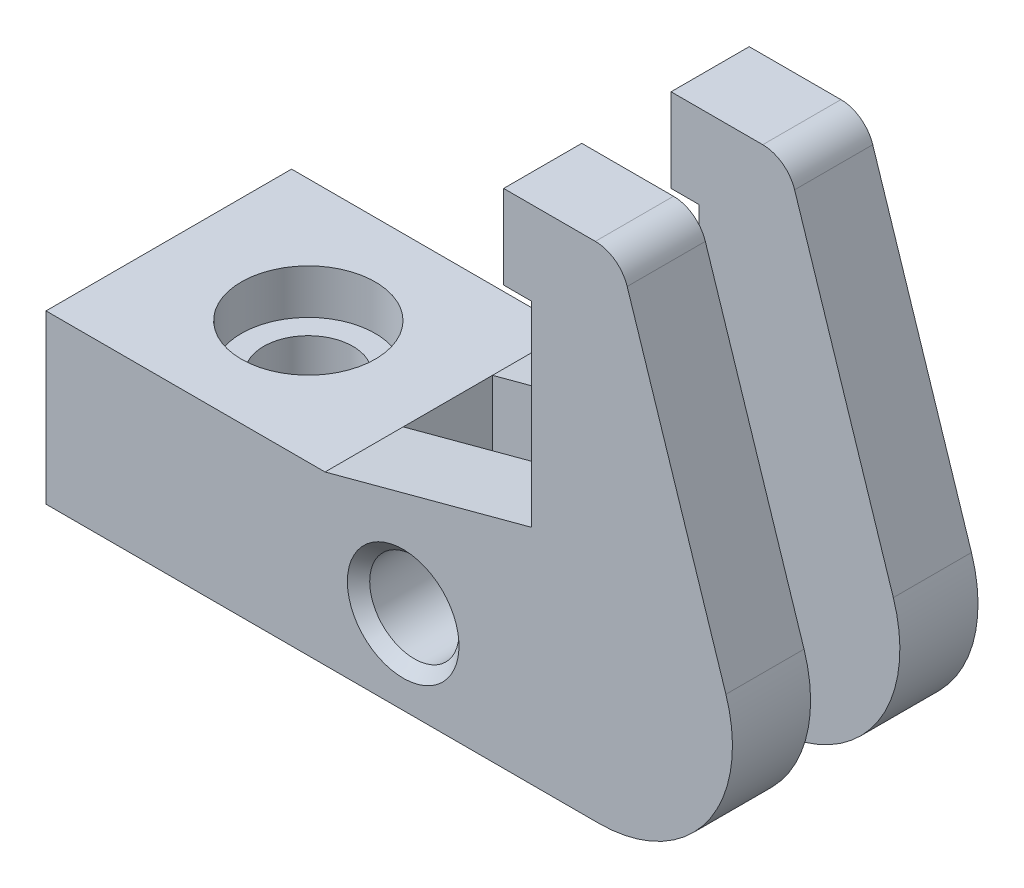
ISO-10303-21;
HEADER;
FILE_DESCRIPTION(('STEP AP214'),'2;1');
FILE_NAME('part.step','',(''),(''),'','','');
FILE_SCHEMA(('AUTOMOTIVE_DESIGN { 1 0 10303 214 1 1 1 1 }'));
ENDSEC;
DATA;
#1=APPLICATION_CONTEXT('core data for automotive mechanical design processes');
#2=APPLICATION_PROTOCOL_DEFINITION('international standard','automotive_design',2000,#1);
#3=PRODUCT_CONTEXT('',#1,'mechanical');
#4=PRODUCT('Part','Part','',(#3));
#5=PRODUCT_RELATED_PRODUCT_CATEGORY('part','',(#4));
#6=PRODUCT_DEFINITION_FORMATION('','',#4);
#7=PRODUCT_DEFINITION_CONTEXT('part definition',#1,'design');
#8=PRODUCT_DEFINITION('design','',#6,#7);
#9=PRODUCT_DEFINITION_SHAPE('','',#8);
#10=(LENGTH_UNIT() NAMED_UNIT(*) SI_UNIT(.MILLI.,.METRE.));
#11=(NAMED_UNIT(*) PLANE_ANGLE_UNIT() SI_UNIT($,.RADIAN.));
#12=(NAMED_UNIT(*) SI_UNIT($,.STERADIAN.) SOLID_ANGLE_UNIT());
#13=UNCERTAINTY_MEASURE_WITH_UNIT(LENGTH_MEASURE(1.E-05),#10,'distance_accuracy_value','');
#14=(GEOMETRIC_REPRESENTATION_CONTEXT(3) GLOBAL_UNCERTAINTY_ASSIGNED_CONTEXT((#13)) GLOBAL_UNIT_ASSIGNED_CONTEXT((#10,
#11,#12)) REPRESENTATION_CONTEXT('',''));
#15=CARTESIAN_POINT('',(0.,0.,0.));
#16=DIRECTION('',(0.,0.,1.));
#17=DIRECTION('',(1.,0.,0.));
#18=AXIS2_PLACEMENT_3D('',#15,#16,#17);
#19=CARTESIAN_POINT('',(32.,0.,11.));
#20=DIRECTION('',(0.,1.,0.));
#21=DIRECTION('',(0.,0.,1.));
#22=AXIS2_PLACEMENT_3D('',#19,#20,#21);
#23=PLANE('',#22);
#24=CARTESIAN_POINT('',(12.5,0.,0.));
#25=DIRECTION('',(0.,1.,0.));
#26=DIRECTION('',(0.,0.,1.));
#27=AXIS2_PLACEMENT_3D('',#24,#25,#26);
#28=CIRCLE('',#27,4.00000000000001);
#29=CARTESIAN_POINT('',(12.5,0.,4.00000000000001));
#30=VERTEX_POINT('',#29);
#31=EDGE_CURVE('E459',#30,#30,#28,.T.);
#32=ORIENTED_EDGE('',*,*,#31,.T.);
#33=EDGE_LOOP('',(#32));
#34=FACE_BOUND('',#33,.T.);
#35=DIRECTION('',(1.,0.,0.));
#36=VECTOR('',#35,1.);
#37=CARTESIAN_POINT('',(25.,0.,4.));
#38=LINE('',#37,#36);
#39=CARTESIAN_POINT('',(25.,0.,4.));
#40=VERTEX_POINT('',#39);
#41=CARTESIAN_POINT('',(49.5,0.,4.));
#42=VERTEX_POINT('',#41);
#43=EDGE_CURVE('E309',#40,#42,#38,.T.);
#44=ORIENTED_EDGE('',*,*,#43,.T.);
#45=DIRECTION('',(0.,0.,-1.));
#46=VECTOR('',#45,1.);
#47=CARTESIAN_POINT('',(49.5,0.,11.));
#48=LINE('',#47,#46);
#49=CARTESIAN_POINT('',(49.5,0.,11.));
#50=VERTEX_POINT('',#49);
#51=EDGE_CURVE('E235',#50,#42,#48,.T.);
#52=ORIENTED_EDGE('',*,*,#51,.F.);
#53=DIRECTION('',(1.,0.,0.));
#54=VECTOR('',#53,1.);
#55=CARTESIAN_POINT('',(0.,0.,11.));
#56=LINE('',#55,#54);
#57=CARTESIAN_POINT('',(0.,0.,11.));
#58=VERTEX_POINT('',#57);
#59=EDGE_CURVE('E118',#58,#50,#56,.T.);
#60=ORIENTED_EDGE('',*,*,#59,.F.);
#61=DIRECTION('',(0.,0.,-1.));
#62=VECTOR('',#61,1.);
#63=CARTESIAN_POINT('',(0.,0.,11.));
#64=LINE('',#63,#62);
#65=CARTESIAN_POINT('',(0.,0.,-11.));
#66=VERTEX_POINT('',#65);
#67=EDGE_CURVE('E234',#58,#66,#64,.T.);
#68=ORIENTED_EDGE('',*,*,#67,.T.);
#69=DIRECTION('',(1.,0.,0.));
#70=VECTOR('',#69,1.);
#71=CARTESIAN_POINT('',(32.,0.,-11.));
#72=LINE('',#71,#70);
#73=CARTESIAN_POINT('',(49.5,0.,-11.));
#74=VERTEX_POINT('',#73);
#75=EDGE_CURVE('E171',#66,#74,#72,.T.);
#76=ORIENTED_EDGE('',*,*,#75,.T.);
#77=CARTESIAN_POINT('',(49.5,0.,-4.));
#78=VERTEX_POINT('',#77);
#79=EDGE_CURVE('E231',#78,#74,#48,.T.);
#80=ORIENTED_EDGE('',*,*,#79,.F.);
#81=DIRECTION('',(-1.,0.,0.));
#82=VECTOR('',#81,1.);
#83=CARTESIAN_POINT('',(25.,0.,-4.));
#84=LINE('',#83,#82);
#85=CARTESIAN_POINT('',(25.,0.,-4.));
#86=VERTEX_POINT('',#85);
#87=EDGE_CURVE('E321',#78,#86,#84,.T.);
#88=ORIENTED_EDGE('',*,*,#87,.T.);
#89=DIRECTION('',(0.,0.,1.));
#90=VECTOR('',#89,1.);
#91=CARTESIAN_POINT('',(25.,0.,-4.));
#92=LINE('',#91,#90);
#93=EDGE_CURVE('E314',#86,#40,#92,.T.);
#94=ORIENTED_EDGE('',*,*,#93,.T.);
#95=EDGE_LOOP('',(#44,#52,#60,#68,#76,#80,#88,#94));
#96=FACE_BOUND('',#95,.T.);
#97=ADVANCED_FACE('F41',(#34,#96),#23,.F.);
#98=CARTESIAN_POINT('',(49.5,12.,11.));
#99=DIRECTION('',(0.,0.,-1.));
#100=DIRECTION('',(-1.,0.,0.));
#101=AXIS2_PLACEMENT_3D('',#98,#99,#100);
#102=CYLINDRICAL_SURFACE('',#101,12.);
#103=CARTESIAN_POINT('',(49.5,12.,4.));
#104=DIRECTION('',(0.,0.,-1.));
#105=DIRECTION('',(-1.,0.,0.));
#106=AXIS2_PLACEMENT_3D('',#103,#104,#105);
#107=CIRCLE('',#106,12.);
#108=CARTESIAN_POINT('',(60.9126781955419,15.7082039324993,4.));
#109=VERTEX_POINT('',#108);
#110=EDGE_CURVE('E176',#109,#42,#107,.T.);
#111=ORIENTED_EDGE('',*,*,#110,.F.);
#112=DIRECTION('',(0.,0.,-1.));
#113=VECTOR('',#112,1.);
#114=CARTESIAN_POINT('',(60.9126781955419,15.7082039324993,11.));
#115=LINE('',#114,#113);
#116=CARTESIAN_POINT('',(60.9126781955419,15.7082039324993,11.));
#117=VERTEX_POINT('',#116);
#118=EDGE_CURVE('E227',#117,#109,#115,.T.);
#119=ORIENTED_EDGE('',*,*,#118,.F.);
#120=CARTESIAN_POINT('',(49.5,12.,11.));
#121=DIRECTION('',(0.,0.,1.));
#122=DIRECTION('',(1.,0.,0.));
#123=AXIS2_PLACEMENT_3D('',#120,#121,#122);
#124=CIRCLE('',#123,12.);
#125=EDGE_CURVE('E326',#50,#117,#124,.T.);
#126=ORIENTED_EDGE('',*,*,#125,.F.);
#127=ORIENTED_EDGE('',*,*,#51,.T.);
#128=EDGE_LOOP('',(#111,#119,#126,#127));
#129=FACE_BOUND('',#128,.T.);
#130=ADVANCED_FACE('F266',(#129),#102,.T.);
#131=CARTESIAN_POINT('',(60.9126781955419,15.7082039324993,-4.));
#132=VERTEX_POINT('',#131);
#133=CARTESIAN_POINT('',(60.9126781955419,15.7082039324993,-11.));
#134=VERTEX_POINT('',#133);
#135=EDGE_CURVE('E229',#132,#134,#115,.T.);
#136=ORIENTED_EDGE('',*,*,#135,.F.);
#137=CARTESIAN_POINT('',(49.5,12.,-4.));
#138=DIRECTION('',(0.,0.,1.));
#139=DIRECTION('',(1.,0.,0.));
#140=AXIS2_PLACEMENT_3D('',#137,#138,#139);
#141=CIRCLE('',#140,12.);
#142=EDGE_CURVE('E427',#78,#132,#141,.T.);
#143=ORIENTED_EDGE('',*,*,#142,.F.);
#144=ORIENTED_EDGE('',*,*,#79,.T.);
#145=CARTESIAN_POINT('',(49.5,12.,-11.));
#146=DIRECTION('',(0.,0.,1.));
#147=DIRECTION('',(1.,0.,0.));
#148=AXIS2_PLACEMENT_3D('',#145,#146,#147);
#149=CIRCLE('',#148,12.);
#150=EDGE_CURVE('E177',#74,#134,#149,.T.);
#151=ORIENTED_EDGE('',*,*,#150,.T.);
#152=EDGE_LOOP('',(#136,#143,#144,#151));
#153=FACE_BOUND('',#152,.T.);
#154=ADVANCED_FACE('F273',(#153),#102,.T.);
#155=CARTESIAN_POINT('',(52.0687386800429,42.9270509831248,11.));
#156=DIRECTION('',(-0.951056516295156,-0.309016994374942,0.));
#157=DIRECTION('',(0.309016994374942,-0.951056516295156,0.));
#158=AXIS2_PLACEMENT_3D('',#155,#156,#157);
#159=PLANE('',#158);
#160=DIRECTION('',(0.309016994374942,-0.951056516295155,0.));
#161=VECTOR('',#160,1.);
#162=CARTESIAN_POINT('',(52.0687386800429,42.9270509831248,4.));
#163=LINE('',#162,#161);
#164=CARTESIAN_POINT('',(52.0687386800429,42.9270509831248,4.));
#165=VERTEX_POINT('',#164);
#166=EDGE_CURVE('E370',#165,#109,#163,.T.);
#167=ORIENTED_EDGE('',*,*,#166,.F.);
#168=DIRECTION('',(0.,0.,-1.));
#169=VECTOR('',#168,1.);
#170=CARTESIAN_POINT('',(52.0687386800429,42.9270509831248,11.));
#171=LINE('',#170,#169);
#172=CARTESIAN_POINT('',(52.0687386800429,42.9270509831248,11.));
#173=VERTEX_POINT('',#172);
#174=EDGE_CURVE('E221',#173,#165,#171,.T.);
#175=ORIENTED_EDGE('',*,*,#174,.F.);
#176=DIRECTION('',(-0.309016994374942,0.951056516295155,0.));
#177=VECTOR('',#176,1.);
#178=CARTESIAN_POINT('',(52.0687386800429,42.9270509831248,11.));
#179=LINE('',#178,#177);
#180=EDGE_CURVE('E327',#117,#173,#179,.T.);
#181=ORIENTED_EDGE('',*,*,#180,.F.);
#182=ORIENTED_EDGE('',*,*,#118,.T.);
#183=EDGE_LOOP('',(#167,#175,#181,#182));
#184=FACE_BOUND('',#183,.T.);
#185=ADVANCED_FACE('F374',(#184),#159,.F.);
#186=DIRECTION('',(-0.309016994374942,0.951056516295155,0.));
#187=VECTOR('',#186,1.);
#188=CARTESIAN_POINT('',(52.0687386800429,42.9270509831248,-4.));
#189=LINE('',#188,#187);
#190=CARTESIAN_POINT('',(52.0687386800429,42.9270509831248,-4.));
#191=VERTEX_POINT('',#190);
#192=EDGE_CURVE('E430',#132,#191,#189,.T.);
#193=ORIENTED_EDGE('',*,*,#192,.F.);
#194=ORIENTED_EDGE('',*,*,#135,.T.);
#195=DIRECTION('',(-0.309016994374942,0.951056516295155,0.));
#196=VECTOR('',#195,1.);
#197=CARTESIAN_POINT('',(52.0687386800429,42.9270509831248,-11.));
#198=LINE('',#197,#196);
#199=CARTESIAN_POINT('',(52.0687386800429,42.9270509831248,-11.));
#200=VERTEX_POINT('',#199);
#201=EDGE_CURVE('E185',#134,#200,#198,.T.);
#202=ORIENTED_EDGE('',*,*,#201,.T.);
#203=EDGE_CURVE('E224',#191,#200,#171,.T.);
#204=ORIENTED_EDGE('',*,*,#203,.F.);
#205=EDGE_LOOP('',(#193,#194,#202,#204));
#206=FACE_BOUND('',#205,.T.);
#207=ADVANCED_FACE('F444',(#206),#159,.F.);
#208=CARTESIAN_POINT('',(49.2155691311574,42.,11.));
#209=DIRECTION('',(0.,0.,-1.));
#210=DIRECTION('',(-1.,0.,0.));
#211=AXIS2_PLACEMENT_3D('',#208,#209,#210);
#212=CYLINDRICAL_SURFACE('',#211,3.);
#213=CARTESIAN_POINT('',(49.2155691311574,42.,4.));
#214=DIRECTION('',(0.,0.,-1.));
#215=DIRECTION('',(-1.,0.,0.));
#216=AXIS2_PLACEMENT_3D('',#213,#214,#215);
#217=CIRCLE('',#216,3.);
#218=CARTESIAN_POINT('',(49.2155691311574,45.,4.));
#219=VERTEX_POINT('',#218);
#220=EDGE_CURVE('E365',#219,#165,#217,.T.);
#221=ORIENTED_EDGE('',*,*,#220,.F.);
#222=DIRECTION('',(0.,0.,-1.));
#223=VECTOR('',#222,1.);
#224=CARTESIAN_POINT('',(49.2155691311574,45.,11.));
#225=LINE('',#224,#223);
#226=CARTESIAN_POINT('',(49.2155691311574,45.,11.));
#227=VERTEX_POINT('',#226);
#228=EDGE_CURVE('E219',#227,#219,#225,.T.);
#229=ORIENTED_EDGE('',*,*,#228,.F.);
#230=CARTESIAN_POINT('',(49.2155691311574,42.,11.));
#231=DIRECTION('',(0.,0.,1.));
#232=DIRECTION('',(-1.,0.,0.));
#233=AXIS2_PLACEMENT_3D('',#230,#231,#232);
#234=CIRCLE('',#233,3.);
#235=EDGE_CURVE('E329',#173,#227,#234,.T.);
#236=ORIENTED_EDGE('',*,*,#235,.F.);
#237=ORIENTED_EDGE('',*,*,#174,.T.);
#238=EDGE_LOOP('',(#221,#229,#236,#237));
#239=FACE_BOUND('',#238,.T.);
#240=ADVANCED_FACE('F378',(#239),#212,.T.);
#241=CARTESIAN_POINT('',(49.2155691311574,42.,-4.));
#242=DIRECTION('',(0.,0.,1.));
#243=DIRECTION('',(1.,0.,0.));
#244=AXIS2_PLACEMENT_3D('',#241,#242,#243);
#245=CIRCLE('',#244,3.);
#246=CARTESIAN_POINT('',(49.2155691311574,45.,-4.));
#247=VERTEX_POINT('',#246);
#248=EDGE_CURVE('E422',#191,#247,#245,.T.);
#249=ORIENTED_EDGE('',*,*,#248,.F.);
#250=ORIENTED_EDGE('',*,*,#203,.T.);
#251=CARTESIAN_POINT('',(49.2155691311574,42.,-11.));
#252=DIRECTION('',(0.,0.,1.));
#253=DIRECTION('',(-1.,0.,0.));
#254=AXIS2_PLACEMENT_3D('',#251,#252,#253);
#255=CIRCLE('',#254,3.);
#256=CARTESIAN_POINT('',(49.2155691311574,45.,-11.));
#257=VERTEX_POINT('',#256);
#258=EDGE_CURVE('E183',#200,#257,#255,.T.);
#259=ORIENTED_EDGE('',*,*,#258,.T.);
#260=EDGE_CURVE('E218',#247,#257,#225,.T.);
#261=ORIENTED_EDGE('',*,*,#260,.F.);
#262=EDGE_LOOP('',(#249,#250,#259,#261));
#263=FACE_BOUND('',#262,.T.);
#264=ADVANCED_FACE('F450',(#263),#212,.T.);
#265=CARTESIAN_POINT('',(41.,45.,11.));
#266=DIRECTION('',(0.,-1.,0.));
#267=DIRECTION('',(1.,0.,0.));
#268=AXIS2_PLACEMENT_3D('',#265,#266,#267);
#269=PLANE('',#268);
#270=DIRECTION('',(1.,0.,0.));
#271=VECTOR('',#270,1.);
#272=CARTESIAN_POINT('',(25.,45.,4.));
#273=LINE('',#272,#271);
#274=CARTESIAN_POINT('',(41.,45.,4.));
#275=VERTEX_POINT('',#274);
#276=EDGE_CURVE('E369',#275,#219,#273,.T.);
#277=ORIENTED_EDGE('',*,*,#276,.F.);
#278=DIRECTION('',(0.,0.,-1.));
#279=VECTOR('',#278,1.);
#280=CARTESIAN_POINT('',(41.,45.,11.));
#281=LINE('',#280,#279);
#282=CARTESIAN_POINT('',(41.,45.,11.));
#283=VERTEX_POINT('',#282);
#284=EDGE_CURVE('E216',#283,#275,#281,.T.);
#285=ORIENTED_EDGE('',*,*,#284,.F.);
#286=DIRECTION('',(-1.,0.,0.));
#287=VECTOR('',#286,1.);
#288=CARTESIAN_POINT('',(41.,45.,11.));
#289=LINE('',#288,#287);
#290=EDGE_CURVE('E338',#227,#283,#289,.T.);
#291=ORIENTED_EDGE('',*,*,#290,.F.);
#292=ORIENTED_EDGE('',*,*,#228,.T.);
#293=EDGE_LOOP('',(#277,#285,#291,#292));
#294=FACE_BOUND('',#293,.T.);
#295=ADVANCED_FACE('F379',(#294),#269,.F.);
#296=DIRECTION('',(-1.,0.,0.));
#297=VECTOR('',#296,1.);
#298=CARTESIAN_POINT('',(25.,45.,-4.));
#299=LINE('',#298,#297);
#300=CARTESIAN_POINT('',(41.,45.,-4.));
#301=VERTEX_POINT('',#300);
#302=EDGE_CURVE('E416',#247,#301,#299,.T.);
#303=ORIENTED_EDGE('',*,*,#302,.F.);
#304=ORIENTED_EDGE('',*,*,#260,.T.);
#305=DIRECTION('',(-1.,0.,0.));
#306=VECTOR('',#305,1.);
#307=CARTESIAN_POINT('',(41.,45.,-11.));
#308=LINE('',#307,#306);
#309=CARTESIAN_POINT('',(41.,45.,-11.));
#310=VERTEX_POINT('',#309);
#311=EDGE_CURVE('E187',#257,#310,#308,.T.);
#312=ORIENTED_EDGE('',*,*,#311,.T.);
#313=EDGE_CURVE('E214',#301,#310,#281,.T.);
#314=ORIENTED_EDGE('',*,*,#313,.F.);
#315=EDGE_LOOP('',(#303,#304,#312,#314));
#316=FACE_BOUND('',#315,.T.);
#317=ADVANCED_FACE('F452',(#316),#269,.F.);
#318=CARTESIAN_POINT('',(41.,37.5,11.));
#319=DIRECTION('',(1.,0.,0.));
#320=DIRECTION('',(0.,0.,-1.));
#321=AXIS2_PLACEMENT_3D('',#318,#319,#320);
#322=PLANE('',#321);
#323=DIRECTION('',(0.,1.,0.));
#324=VECTOR('',#323,1.);
#325=CARTESIAN_POINT('',(41.,37.5,4.));
#326=LINE('',#325,#324);
#327=CARTESIAN_POINT('',(41.,37.5,4.));
#328=VERTEX_POINT('',#327);
#329=EDGE_CURVE('E346',#328,#275,#326,.T.);
#330=ORIENTED_EDGE('',*,*,#329,.F.);
#331=DIRECTION('',(0.,0.,-1.));
#332=VECTOR('',#331,1.);
#333=CARTESIAN_POINT('',(41.,37.5,11.));
#334=LINE('',#333,#332);
#335=CARTESIAN_POINT('',(41.,37.5,11.));
#336=VERTEX_POINT('',#335);
#337=EDGE_CURVE('E215',#336,#328,#334,.T.);
#338=ORIENTED_EDGE('',*,*,#337,.F.);
#339=DIRECTION('',(0.,-1.,0.));
#340=VECTOR('',#339,1.);
#341=CARTESIAN_POINT('',(41.,37.5,11.));
#342=LINE('',#341,#340);
#343=EDGE_CURVE('E337',#283,#336,#342,.T.);
#344=ORIENTED_EDGE('',*,*,#343,.F.);
#345=ORIENTED_EDGE('',*,*,#284,.T.);
#346=EDGE_LOOP('',(#330,#338,#344,#345));
#347=FACE_BOUND('',#346,.T.);
#348=ADVANCED_FACE('F344',(#347),#322,.F.);
#349=DIRECTION('',(0.,-1.,0.));
#350=VECTOR('',#349,1.);
#351=CARTESIAN_POINT('',(41.,37.5,-4.));
#352=LINE('',#351,#350);
#353=CARTESIAN_POINT('',(41.,37.5,-4.));
#354=VERTEX_POINT('',#353);
#355=EDGE_CURVE('E421',#301,#354,#352,.T.);
#356=ORIENTED_EDGE('',*,*,#355,.F.);
#357=ORIENTED_EDGE('',*,*,#313,.T.);
#358=DIRECTION('',(0.,-1.,0.));
#359=VECTOR('',#358,1.);
#360=CARTESIAN_POINT('',(41.,37.5,-11.));
#361=LINE('',#360,#359);
#362=CARTESIAN_POINT('',(41.,37.5,-11.));
#363=VERTEX_POINT('',#362);
#364=EDGE_CURVE('E191',#310,#363,#361,.T.);
#365=ORIENTED_EDGE('',*,*,#364,.T.);
#366=EDGE_CURVE('E211',#354,#363,#334,.T.);
#367=ORIENTED_EDGE('',*,*,#366,.F.);
#368=EDGE_LOOP('',(#356,#357,#365,#367));
#369=FACE_BOUND('',#368,.T.);
#370=ADVANCED_FACE('F496',(#369),#322,.F.);
#371=CARTESIAN_POINT('',(43.5,37.5,11.));
#372=DIRECTION('',(0.,1.,0.));
#373=DIRECTION('',(0.,0.,1.));
#374=AXIS2_PLACEMENT_3D('',#371,#372,#373);
#375=PLANE('',#374);
#376=DIRECTION('',(-1.,0.,0.));
#377=VECTOR('',#376,1.);
#378=CARTESIAN_POINT('',(43.5,37.5,4.));
#379=LINE('',#378,#377);
#380=CARTESIAN_POINT('',(43.5,37.5,4.));
#381=VERTEX_POINT('',#380);
#382=EDGE_CURVE('E355',#381,#328,#379,.T.);
#383=ORIENTED_EDGE('',*,*,#382,.F.);
#384=DIRECTION('',(0.,0.,-1.));
#385=VECTOR('',#384,1.);
#386=CARTESIAN_POINT('',(43.5,37.5,11.));
#387=LINE('',#386,#385);
#388=CARTESIAN_POINT('',(43.5,37.5,11.));
#389=VERTEX_POINT('',#388);
#390=EDGE_CURVE('E207',#389,#381,#387,.T.);
#391=ORIENTED_EDGE('',*,*,#390,.F.);
#392=DIRECTION('',(1.,0.,0.));
#393=VECTOR('',#392,1.);
#394=CARTESIAN_POINT('',(43.5,37.5,11.));
#395=LINE('',#394,#393);
#396=EDGE_CURVE('E150',#336,#389,#395,.T.);
#397=ORIENTED_EDGE('',*,*,#396,.F.);
#398=ORIENTED_EDGE('',*,*,#337,.T.);
#399=EDGE_LOOP('',(#383,#391,#397,#398));
#400=FACE_BOUND('',#399,.T.);
#401=ADVANCED_FACE('F353',(#400),#375,.F.);
#402=DIRECTION('',(1.,0.,0.));
#403=VECTOR('',#402,1.);
#404=CARTESIAN_POINT('',(43.5,37.5,-4.));
#405=LINE('',#404,#403);
#406=CARTESIAN_POINT('',(43.5,37.5,-4.));
#407=VERTEX_POINT('',#406);
#408=EDGE_CURVE('E418',#354,#407,#405,.T.);
#409=ORIENTED_EDGE('',*,*,#408,.F.);
#410=ORIENTED_EDGE('',*,*,#366,.T.);
#411=DIRECTION('',(1.,0.,0.));
#412=VECTOR('',#411,1.);
#413=CARTESIAN_POINT('',(43.5,37.5,-11.));
#414=LINE('',#413,#412);
#415=CARTESIAN_POINT('',(43.5,37.5,-11.));
#416=VERTEX_POINT('',#415);
#417=EDGE_CURVE('E192',#363,#416,#414,.T.);
#418=ORIENTED_EDGE('',*,*,#417,.T.);
#419=EDGE_CURVE('E161',#407,#416,#387,.T.);
#420=ORIENTED_EDGE('',*,*,#419,.F.);
#421=EDGE_LOOP('',(#409,#410,#418,#420));
#422=FACE_BOUND('',#421,.T.);
#423=ADVANCED_FACE('F497',(#422),#375,.F.);
#424=CARTESIAN_POINT('',(43.5,19.9570600599758,11.));
#425=DIRECTION('',(1.,0.,0.));
#426=DIRECTION('',(0.,0.,-1.));
#427=AXIS2_PLACEMENT_3D('',#424,#425,#426);
#428=PLANE('',#427);
#429=DIRECTION('',(0.,1.,0.));
#430=VECTOR('',#429,1.);
#431=CARTESIAN_POINT('',(43.5,19.9570600599758,4.));
#432=LINE('',#431,#430);
#433=CARTESIAN_POINT('',(43.5,19.9570600599758,4.));
#434=VERTEX_POINT('',#433);
#435=EDGE_CURVE('E158',#434,#381,#432,.T.);
#436=ORIENTED_EDGE('',*,*,#435,.F.);
#437=DIRECTION('',(0.,0.,-1.));
#438=VECTOR('',#437,1.);
#439=CARTESIAN_POINT('',(43.5,19.9570600599758,11.));
#440=LINE('',#439,#438);
#441=CARTESIAN_POINT('',(43.5,19.9570600599758,11.));
#442=VERTEX_POINT('',#441);
#443=EDGE_CURVE('E152',#442,#434,#440,.T.);
#444=ORIENTED_EDGE('',*,*,#443,.F.);
#445=DIRECTION('',(0.,-1.,0.));
#446=VECTOR('',#445,1.);
#447=CARTESIAN_POINT('',(43.5,19.9570600599758,11.));
#448=LINE('',#447,#446);
#449=EDGE_CURVE('E139',#389,#442,#448,.T.);
#450=ORIENTED_EDGE('',*,*,#449,.F.);
#451=ORIENTED_EDGE('',*,*,#390,.T.);
#452=EDGE_LOOP('',(#436,#444,#450,#451));
#453=FACE_BOUND('',#452,.T.);
#454=ADVANCED_FACE('F154',(#453),#428,.F.);
#455=DIRECTION('',(0.,-1.,0.));
#456=VECTOR('',#455,1.);
#457=CARTESIAN_POINT('',(43.5,19.9570600599758,-4.));
#458=LINE('',#457,#456);
#459=CARTESIAN_POINT('',(43.5,19.9570600599758,-4.));
#460=VERTEX_POINT('',#459);
#461=EDGE_CURVE('E412',#407,#460,#458,.T.);
#462=ORIENTED_EDGE('',*,*,#461,.F.);
#463=ORIENTED_EDGE('',*,*,#419,.T.);
#464=DIRECTION('',(0.,-1.,0.));
#465=VECTOR('',#464,1.);
#466=CARTESIAN_POINT('',(43.5,19.9570600599758,-11.));
#467=LINE('',#466,#465);
#468=CARTESIAN_POINT('',(43.5,19.9570600599758,-11.));
#469=VERTEX_POINT('',#468);
#470=EDGE_CURVE('E197',#416,#469,#467,.T.);
#471=ORIENTED_EDGE('',*,*,#470,.T.);
#472=EDGE_CURVE('E165',#460,#469,#440,.T.);
#473=ORIENTED_EDGE('',*,*,#472,.F.);
#474=EDGE_LOOP('',(#462,#463,#471,#473));
#475=FACE_BOUND('',#474,.T.);
#476=ADVANCED_FACE('F492',(#475),#428,.F.);
#477=CARTESIAN_POINT('',(25.,15.,11.));
#478=DIRECTION('',(0.258819045102522,-0.965925826289068,0.));
#479=DIRECTION('',(0.965925826289068,0.258819045102522,0.));
#480=AXIS2_PLACEMENT_3D('',#477,#478,#479);
#481=PLANE('',#480);
#482=DIRECTION('',(0.965925826289068,0.258819045102522,0.));
#483=VECTOR('',#482,1.);
#484=CARTESIAN_POINT('',(25.,15.,4.));
#485=LINE('',#484,#483);
#486=CARTESIAN_POINT('',(25.,15.,4.));
#487=VERTEX_POINT('',#486);
#488=EDGE_CURVE('E239',#487,#434,#485,.T.);
#489=ORIENTED_EDGE('',*,*,#488,.F.);
#490=DIRECTION('',(0.,0.,-1.));
#491=VECTOR('',#490,1.);
#492=CARTESIAN_POINT('',(25.,15.,11.));
#493=LINE('',#492,#491);
#494=CARTESIAN_POINT('',(25.,15.,11.));
#495=VERTEX_POINT('',#494);
#496=EDGE_CURVE('E167',#495,#487,#493,.T.);
#497=ORIENTED_EDGE('',*,*,#496,.F.);
#498=DIRECTION('',(-0.965925826289068,-0.258819045102522,0.));
#499=VECTOR('',#498,1.);
#500=CARTESIAN_POINT('',(25.,15.,11.));
#501=LINE('',#500,#499);
#502=EDGE_CURVE('E145',#442,#495,#501,.T.);
#503=ORIENTED_EDGE('',*,*,#502,.F.);
#504=ORIENTED_EDGE('',*,*,#443,.T.);
#505=EDGE_LOOP('',(#489,#497,#503,#504));
#506=FACE_BOUND('',#505,.T.);
#507=ADVANCED_FACE('F163',(#506),#481,.F.);
#508=DIRECTION('',(-0.965925826289068,-0.258819045102522,0.));
#509=VECTOR('',#508,1.);
#510=CARTESIAN_POINT('',(25.,15.,-4.));
#511=LINE('',#510,#509);
#512=CARTESIAN_POINT('',(25.,15.,-4.));
#513=VERTEX_POINT('',#512);
#514=EDGE_CURVE('E240',#460,#513,#511,.T.);
#515=ORIENTED_EDGE('',*,*,#514,.F.);
#516=ORIENTED_EDGE('',*,*,#472,.T.);
#517=DIRECTION('',(-0.965925826289068,-0.258819045102522,0.));
#518=VECTOR('',#517,1.);
#519=CARTESIAN_POINT('',(25.,15.,-11.));
#520=LINE('',#519,#518);
#521=CARTESIAN_POINT('',(25.,15.,-11.));
#522=VERTEX_POINT('',#521);
#523=EDGE_CURVE('E199',#469,#522,#520,.T.);
#524=ORIENTED_EDGE('',*,*,#523,.T.);
#525=EDGE_CURVE('E206',#513,#522,#493,.T.);
#526=ORIENTED_EDGE('',*,*,#525,.F.);
#527=EDGE_LOOP('',(#515,#516,#524,#526));
#528=FACE_BOUND('',#527,.T.);
#529=ADVANCED_FACE('F282',(#528),#481,.F.);
#530=CARTESIAN_POINT('',(0.,0.,11.));
#531=DIRECTION('',(1.,0.,0.));
#532=DIRECTION('',(0.,0.,-1.));
#533=AXIS2_PLACEMENT_3D('',#530,#531,#532);
#534=PLANE('',#533);
#535=DIRECTION('',(0.,-1.,0.));
#536=VECTOR('',#535,1.);
#537=CARTESIAN_POINT('',(0.,0.,-11.));
#538=LINE('',#537,#536);
#539=CARTESIAN_POINT('',(0.,15.,-11.));
#540=VERTEX_POINT('',#539);
#541=EDGE_CURVE('E174',#540,#66,#538,.T.);
#542=ORIENTED_EDGE('',*,*,#541,.T.);
#543=ORIENTED_EDGE('',*,*,#67,.F.);
#544=DIRECTION('',(0.,-1.,0.));
#545=VECTOR('',#544,1.);
#546=CARTESIAN_POINT('',(0.,0.,11.));
#547=LINE('',#546,#545);
#548=CARTESIAN_POINT('',(0.,15.,11.));
#549=VERTEX_POINT('',#548);
#550=EDGE_CURVE('E204',#549,#58,#547,.T.);
#551=ORIENTED_EDGE('',*,*,#550,.F.);
#552=DIRECTION('',(0.,0.,-1.));
#553=VECTOR('',#552,1.);
#554=CARTESIAN_POINT('',(0.,15.,11.));
#555=LINE('',#554,#553);
#556=EDGE_CURVE('E169',#549,#540,#555,.T.);
#557=ORIENTED_EDGE('',*,*,#556,.T.);
#558=EDGE_LOOP('',(#542,#543,#551,#557));
#559=FACE_BOUND('',#558,.T.);
#560=ADVANCED_FACE('F278',(#559),#534,.F.);
#561=CARTESIAN_POINT('',(0.,15.,11.));
#562=DIRECTION('',(0.,-1.,0.));
#563=DIRECTION('',(0.,0.,-1.));
#564=AXIS2_PLACEMENT_3D('',#561,#562,#563);
#565=PLANE('',#564);
#566=CARTESIAN_POINT('',(12.5,15.,0.));
#567=DIRECTION('',(0.,1.,0.));
#568=DIRECTION('',(0.,0.,1.));
#569=AXIS2_PLACEMENT_3D('',#566,#567,#568);
#570=CIRCLE('',#569,6.00000000000001);
#571=CARTESIAN_POINT('',(12.5,15.,6.00000000000001));
#572=VERTEX_POINT('',#571);
#573=EDGE_CURVE('E468',#572,#572,#570,.T.);
#574=ORIENTED_EDGE('',*,*,#573,.F.);
#575=EDGE_LOOP('',(#574));
#576=FACE_BOUND('',#575,.T.);
#577=DIRECTION('',(-1.,0.,0.));
#578=VECTOR('',#577,1.);
#579=CARTESIAN_POINT('',(0.,15.,-11.));
#580=LINE('',#579,#578);
#581=EDGE_CURVE('E110',#522,#540,#580,.T.);
#582=ORIENTED_EDGE('',*,*,#581,.T.);
#583=ORIENTED_EDGE('',*,*,#556,.F.);
#584=DIRECTION('',(-1.,0.,0.));
#585=VECTOR('',#584,1.);
#586=CARTESIAN_POINT('',(0.,15.,11.));
#587=LINE('',#586,#585);
#588=EDGE_CURVE('E66',#495,#549,#587,.T.);
#589=ORIENTED_EDGE('',*,*,#588,.F.);
#590=ORIENTED_EDGE('',*,*,#496,.T.);
#591=EDGE_CURVE('E210',#487,#513,#493,.T.);
#592=ORIENTED_EDGE('',*,*,#591,.T.);
#593=ORIENTED_EDGE('',*,*,#525,.T.);
#594=EDGE_LOOP('',(#582,#583,#589,#590,#592,#593));
#595=FACE_BOUND('',#594,.T.);
#596=ADVANCED_FACE('F284',(#576,#595),#565,.F.);
#597=CARTESIAN_POINT('',(49.2155691311574,42.,11.));
#598=DIRECTION('',(0.,0.,-1.));
#599=DIRECTION('',(-1.,0.,0.));
#600=AXIS2_PLACEMENT_3D('',#597,#598,#599);
#601=PLANE('',#600);
#602=CARTESIAN_POINT('',(32.,7.5,11.));
#603=DIRECTION('',(0.,0.,-1.));
#604=DIRECTION('',(-1.,0.,0.));
#605=AXIS2_PLACEMENT_3D('',#602,#603,#604);
#606=CIRCLE('',#605,5.00000000000002);
#607=CARTESIAN_POINT('',(27.,7.5,11.));
#608=VERTEX_POINT('',#607);
#609=EDGE_CURVE('E11',#608,#608,#606,.T.);
#610=ORIENTED_EDGE('',*,*,#609,.T.);
#611=EDGE_LOOP('',(#610));
#612=FACE_BOUND('',#611,.T.);
#613=ORIENTED_EDGE('',*,*,#550,.T.);
#614=ORIENTED_EDGE('',*,*,#59,.T.);
#615=ORIENTED_EDGE('',*,*,#125,.T.);
#616=ORIENTED_EDGE('',*,*,#180,.T.);
#617=ORIENTED_EDGE('',*,*,#235,.T.);
#618=ORIENTED_EDGE('',*,*,#290,.T.);
#619=ORIENTED_EDGE('',*,*,#343,.T.);
#620=ORIENTED_EDGE('',*,*,#396,.T.);
#621=ORIENTED_EDGE('',*,*,#449,.T.);
#622=ORIENTED_EDGE('',*,*,#502,.T.);
#623=ORIENTED_EDGE('',*,*,#588,.T.);
#624=EDGE_LOOP('',(#613,#614,#615,#616,#617,#618,#619,#620,#621,#622,#623));
#625=FACE_BOUND('',#624,.T.);
#626=ADVANCED_FACE('F142',(#612,#625),#601,.F.);
#627=CARTESIAN_POINT('',(49.2155691311574,42.,-11.));
#628=DIRECTION('',(0.,0.,-1.));
#629=DIRECTION('',(-1.,0.,0.));
#630=AXIS2_PLACEMENT_3D('',#627,#628,#629);
#631=PLANE('',#630);
#632=CARTESIAN_POINT('',(32.,7.5,-11.));
#633=DIRECTION('',(0.,0.,-1.));
#634=DIRECTION('',(-1.,0.,0.));
#635=AXIS2_PLACEMENT_3D('',#632,#633,#634);
#636=CIRCLE('',#635,5.);
#637=CARTESIAN_POINT('',(27.,7.5,-11.));
#638=VERTEX_POINT('',#637);
#639=EDGE_CURVE('E244',#638,#638,#636,.F.);
#640=ORIENTED_EDGE('',*,*,#639,.T.);
#641=EDGE_LOOP('',(#640));
#642=FACE_BOUND('',#641,.T.);
#643=ORIENTED_EDGE('',*,*,#541,.F.);
#644=ORIENTED_EDGE('',*,*,#581,.F.);
#645=ORIENTED_EDGE('',*,*,#523,.F.);
#646=ORIENTED_EDGE('',*,*,#470,.F.);
#647=ORIENTED_EDGE('',*,*,#417,.F.);
#648=ORIENTED_EDGE('',*,*,#364,.F.);
#649=ORIENTED_EDGE('',*,*,#311,.F.);
#650=ORIENTED_EDGE('',*,*,#258,.F.);
#651=ORIENTED_EDGE('',*,*,#201,.F.);
#652=ORIENTED_EDGE('',*,*,#150,.F.);
#653=ORIENTED_EDGE('',*,*,#75,.F.);
#654=EDGE_LOOP('',(#643,#644,#645,#646,#647,#648,#649,#650,#651,#652,#653));
#655=FACE_BOUND('',#654,.T.);
#656=ADVANCED_FACE('F301',(#642,#655),#631,.T.);
#657=CARTESIAN_POINT('',(25.,45.,4.));
#658=DIRECTION('',(0.,0.,-1.));
#659=DIRECTION('',(-1.,0.,0.));
#660=AXIS2_PLACEMENT_3D('',#657,#658,#659);
#661=PLANE('',#660);
#662=CARTESIAN_POINT('',(32.,7.5,4.));
#663=DIRECTION('',(0.,0.,-1.));
#664=DIRECTION('',(-1.,0.,0.));
#665=AXIS2_PLACEMENT_3D('',#662,#663,#664);
#666=CIRCLE('',#665,4.00000000000001);
#667=CARTESIAN_POINT('',(28.,7.5,4.));
#668=VERTEX_POINT('',#667);
#669=EDGE_CURVE('E246',#668,#668,#666,.T.);
#670=ORIENTED_EDGE('',*,*,#669,.F.);
#671=EDGE_LOOP('',(#670));
#672=FACE_BOUND('',#671,.T.);
#673=ORIENTED_EDGE('',*,*,#110,.T.);
#674=ORIENTED_EDGE('',*,*,#43,.F.);
#675=DIRECTION('',(0.,-1.,0.));
#676=VECTOR('',#675,1.);
#677=CARTESIAN_POINT('',(25.,45.,4.));
#678=LINE('',#677,#676);
#679=EDGE_CURVE('E411',#487,#40,#678,.T.);
#680=ORIENTED_EDGE('',*,*,#679,.F.);
#681=ORIENTED_EDGE('',*,*,#488,.T.);
#682=ORIENTED_EDGE('',*,*,#435,.T.);
#683=ORIENTED_EDGE('',*,*,#382,.T.);
#684=ORIENTED_EDGE('',*,*,#329,.T.);
#685=ORIENTED_EDGE('',*,*,#276,.T.);
#686=ORIENTED_EDGE('',*,*,#220,.T.);
#687=ORIENTED_EDGE('',*,*,#166,.T.);
#688=EDGE_LOOP('',(#673,#674,#680,#681,#682,#683,#684,#685,#686,#687));
#689=FACE_BOUND('',#688,.T.);
#690=ADVANCED_FACE('F368',(#672,#689),#661,.T.);
#691=CARTESIAN_POINT('',(25.,45.,-4.));
#692=DIRECTION('',(0.,0.,1.));
#693=DIRECTION('',(1.,0.,0.));
#694=AXIS2_PLACEMENT_3D('',#691,#692,#693);
#695=PLANE('',#694);
#696=CARTESIAN_POINT('',(32.,7.5,-4.));
#697=DIRECTION('',(0.,0.,1.));
#698=DIRECTION('',(1.,0.,0.));
#699=AXIS2_PLACEMENT_3D('',#696,#697,#698);
#700=CIRCLE('',#699,4.00000000000001);
#701=CARTESIAN_POINT('',(36.,7.5,-4.));
#702=VERTEX_POINT('',#701);
#703=EDGE_CURVE('E242',#702,#702,#700,.T.);
#704=ORIENTED_EDGE('',*,*,#703,.F.);
#705=EDGE_LOOP('',(#704));
#706=FACE_BOUND('',#705,.T.);
#707=ORIENTED_EDGE('',*,*,#142,.T.);
#708=ORIENTED_EDGE('',*,*,#192,.T.);
#709=ORIENTED_EDGE('',*,*,#248,.T.);
#710=ORIENTED_EDGE('',*,*,#302,.T.);
#711=ORIENTED_EDGE('',*,*,#355,.T.);
#712=ORIENTED_EDGE('',*,*,#408,.T.);
#713=ORIENTED_EDGE('',*,*,#461,.T.);
#714=ORIENTED_EDGE('',*,*,#514,.T.);
#715=DIRECTION('',(0.,-1.,0.));
#716=VECTOR('',#715,1.);
#717=CARTESIAN_POINT('',(25.,45.,-4.));
#718=LINE('',#717,#716);
#719=EDGE_CURVE('E60',#513,#86,#718,.T.);
#720=ORIENTED_EDGE('',*,*,#719,.T.);
#721=ORIENTED_EDGE('',*,*,#87,.F.);
#722=EDGE_LOOP('',(#707,#708,#709,#710,#711,#712,#713,#714,#720,#721));
#723=FACE_BOUND('',#722,.T.);
#724=ADVANCED_FACE('F440',(#706,#723),#695,.T.);
#725=CARTESIAN_POINT('',(25.,45.,-4.));
#726=DIRECTION('',(1.,0.,0.));
#727=DIRECTION('',(0.,0.,-1.));
#728=AXIS2_PLACEMENT_3D('',#725,#726,#727);
#729=PLANE('',#728);
#730=ORIENTED_EDGE('',*,*,#591,.F.);
#731=ORIENTED_EDGE('',*,*,#679,.T.);
#732=ORIENTED_EDGE('',*,*,#93,.F.);
#733=ORIENTED_EDGE('',*,*,#719,.F.);
#734=EDGE_LOOP('',(#730,#731,#732,#733));
#735=FACE_BOUND('',#734,.T.);
#736=ADVANCED_FACE('F415',(#735),#729,.T.);
#737=CARTESIAN_POINT('',(12.5,15.,0.));
#738=DIRECTION('',(0.,1.,0.));
#739=DIRECTION('',(0.,0.,1.));
#740=AXIS2_PLACEMENT_3D('',#737,#738,#739);
#741=CYLINDRICAL_SURFACE('',#740,4.00000000000001);
#742=ORIENTED_EDGE('',*,*,#31,.F.);
#743=EDGE_LOOP('',(#742));
#744=FACE_BOUND('',#743,.T.);
#745=CARTESIAN_POINT('',(12.5,11.,0.));
#746=DIRECTION('',(0.,1.,0.));
#747=DIRECTION('',(0.,0.,1.));
#748=AXIS2_PLACEMENT_3D('',#745,#746,#747);
#749=CIRCLE('',#748,4.00000000000001);
#750=CARTESIAN_POINT('',(12.5,11.,4.00000000000001));
#751=VERTEX_POINT('',#750);
#752=EDGE_CURVE('E458',#751,#751,#749,.T.);
#753=ORIENTED_EDGE('',*,*,#752,.T.);
#754=EDGE_LOOP('',(#753));
#755=FACE_BOUND('',#754,.T.);
#756=ADVANCED_FACE('F488',(#744,#755),#741,.F.);
#757=CARTESIAN_POINT('',(16.5,11.,0.));
#758=DIRECTION('',(0.,-1.,0.));
#759=DIRECTION('',(0.,0.,-1.));
#760=AXIS2_PLACEMENT_3D('',#757,#758,#759);
#761=PLANE('',#760);
#762=ORIENTED_EDGE('',*,*,#752,.F.);
#763=EDGE_LOOP('',(#762));
#764=FACE_BOUND('',#763,.T.);
#765=CARTESIAN_POINT('',(12.5,11.,0.));
#766=DIRECTION('',(0.,1.,0.));
#767=DIRECTION('',(0.,0.,1.));
#768=AXIS2_PLACEMENT_3D('',#765,#766,#767);
#769=CIRCLE('',#768,6.00000000000002);
#770=CARTESIAN_POINT('',(12.5,11.,6.00000000000002));
#771=VERTEX_POINT('',#770);
#772=EDGE_CURVE('E462',#771,#771,#769,.T.);
#773=ORIENTED_EDGE('',*,*,#772,.T.);
#774=EDGE_LOOP('',(#773));
#775=FACE_BOUND('',#774,.T.);
#776=ADVANCED_FACE('F555',(#764,#775),#761,.F.);
#777=CARTESIAN_POINT('',(12.5,15.,0.));
#778=DIRECTION('',(0.,1.,0.));
#779=DIRECTION('',(0.,0.,1.));
#780=AXIS2_PLACEMENT_3D('',#777,#778,#779);
#781=CYLINDRICAL_SURFACE('',#780,6.00000000000001);
#782=ORIENTED_EDGE('',*,*,#772,.F.);
#783=EDGE_LOOP('',(#782));
#784=FACE_BOUND('',#783,.T.);
#785=ORIENTED_EDGE('',*,*,#573,.T.);
#786=EDGE_LOOP('',(#785));
#787=FACE_BOUND('',#786,.T.);
#788=ADVANCED_FACE('F561',(#784,#787),#781,.F.);
#789=CARTESIAN_POINT('',(32.,7.5,-11.));
#790=DIRECTION('',(0.,0.,1.));
#791=DIRECTION('',(1.,0.,0.));
#792=AXIS2_PLACEMENT_3D('',#789,#790,#791);
#793=CYLINDRICAL_SURFACE('',#792,4.00000000000001);
#794=CARTESIAN_POINT('',(32.,7.5,-10.));
#795=DIRECTION('',(0.,0.,-1.));
#796=DIRECTION('',(-1.,0.,0.));
#797=AXIS2_PLACEMENT_3D('',#794,#795,#796);
#798=CIRCLE('',#797,4.00000000000001);
#799=CARTESIAN_POINT('',(28.,7.5,-10.));
#800=VERTEX_POINT('',#799);
#801=EDGE_CURVE('E247',#800,#800,#798,.T.);
#802=ORIENTED_EDGE('',*,*,#801,.T.);
#803=EDGE_LOOP('',(#802));
#804=FACE_BOUND('',#803,.T.);
#805=ORIENTED_EDGE('',*,*,#703,.T.);
#806=EDGE_LOOP('',(#805));
#807=FACE_BOUND('',#806,.T.);
#808=ADVANCED_FACE('F568',(#804,#807),#793,.F.);
#809=CARTESIAN_POINT('',(32.,7.5,9.99999999999999));
#810=DIRECTION('',(0.,0.,-1.));
#811=DIRECTION('',(-1.,0.,0.));
#812=AXIS2_PLACEMENT_3D('',#809,#810,#811);
#813=CIRCLE('',#812,4.00000000000001);
#814=CARTESIAN_POINT('',(28.,7.5,9.99999999999999));
#815=VERTEX_POINT('',#814);
#816=EDGE_CURVE('E49',#815,#815,#813,.F.);
#817=ORIENTED_EDGE('',*,*,#816,.T.);
#818=EDGE_LOOP('',(#817));
#819=FACE_BOUND('',#818,.T.);
#820=ORIENTED_EDGE('',*,*,#669,.T.);
#821=EDGE_LOOP('',(#820));
#822=FACE_BOUND('',#821,.T.);
#823=ADVANCED_FACE('F255',(#819,#822),#793,.F.);
#824=CARTESIAN_POINT('',(32.,7.5,-11.));
#825=DIRECTION('',(0.,0.,-1.));
#826=DIRECTION('',(-1.,0.,0.));
#827=AXIS2_PLACEMENT_3D('',#824,#825,#826);
#828=CONICAL_SURFACE('',#827,5.,0.785398163397449);
#829=ORIENTED_EDGE('',*,*,#801,.F.);
#830=EDGE_LOOP('',(#829));
#831=FACE_BOUND('',#830,.T.);
#832=ORIENTED_EDGE('',*,*,#639,.F.);
#833=EDGE_LOOP('',(#832));
#834=FACE_BOUND('',#833,.T.);
#835=ADVANCED_FACE('F256',(#831,#834),#828,.F.);
#836=CARTESIAN_POINT('',(32.,7.5,9.99999999999999));
#837=DIRECTION('',(0.,0.,1.));
#838=DIRECTION('',(1.,0.,0.));
#839=AXIS2_PLACEMENT_3D('',#836,#837,#838);
#840=CONICAL_SURFACE('',#839,4.00000000000001,0.78539816339745);
#841=ORIENTED_EDGE('',*,*,#609,.F.);
#842=EDGE_LOOP('',(#841));
#843=FACE_BOUND('',#842,.T.);
#844=ORIENTED_EDGE('',*,*,#816,.F.);
#845=EDGE_LOOP('',(#844));
#846=FACE_BOUND('',#845,.T.);
#847=ADVANCED_FACE('F42',(#843,#846),#840,.F.);
#848=CLOSED_SHELL('',(#97,#130,#154,#185,#207,#240,#264,#295,#317,#348,#370,#401,#423,#454,#476,
#507,#529,#560,#596,#626,#656,#690,#724,#736,#756,#776,#788,#808,#823,#835,#847));
#849=MANIFOLD_SOLID_BREP('B2',#848);
#850=ADVANCED_BREP_SHAPE_REPRESENTATION('',(#18,#849),#14);
#851=SHAPE_DEFINITION_REPRESENTATION(#9,#850);
ENDSEC;
END-ISO-10303-21;
